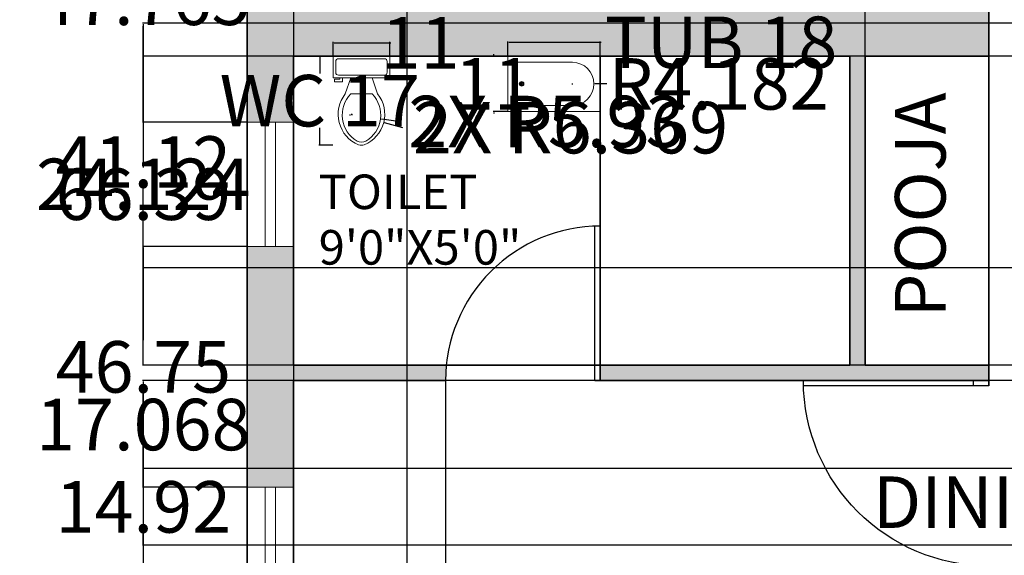
# Model space of a CAD drawing. Units: inches. Extents: x -75 to 484, y -248 to 214.
# Tile 2 of 7: x -29 to 162, y -87 to 17. Entities that reach past the tile are written whole.
import ezdxf

# ---------------------------------------------------------------- set-up
doc = ezdxf.new("R2010")
doc.units = ezdxf.units.IN
doc.header["$MEASUREMENT"] = 0
doc.linetypes.add('ACAD_ISO02W100', pattern=[15, 12, -3])
for name, color, linetype, lineweight in [('A-ANNO-DIMS', 2, 'Continuous', 18), ('A-AREA-IDEN', 7, 'Continuous', 18), ('A-DOOR', 3, 'Continuous', 25), ('A-FLOR-FIXT', 8, 'Continuous', 18), ('A-GLAZ', 4, 'Continuous', 18), ('A-WALL', 7, 'Continuous', 35), ('A-WALL-OVHD', 7, 'ACAD_ISO02W100', 18)]:
    doc.layers.add(name, color=color, linetype=linetype, lineweight=lineweight)
doc.layers.add('A-WALL-PATT', color=252, linetype='Continuous', lineweight=9, true_color=0x939598)
doc.styles.get("Standard").update_dxf_attribs({"font": 'arial.ttf'})
doc.dimstyles.get("Standard").update_dxf_attribs({"dimtxt": 10, "dimasz": 0.18, "dimexe": 0.18, "dimexo": 0.0625, "dimgap": 0.09, "dimtad": 0, "dimtih": 1, "dimtoh": 1, "dimdec": 0, "dimzin": 0, "dimdsep": 46, "dimlunit": 3, "dimtxsty": 'Standard', "dimcen": 0.09, "dimadec": 0, "dimazin": 0, "dimtfac": 1, "dimtdec": 0, "dimtofl": 0, "dimtmove": 0, "dimatfit": 3, "dimfxl": 1, "dimtolj": 1, "dimtzin": 0, "dimarcsym": 0})

# ---------------------------------------------------------------- blocks, each defined once
blk = doc.blocks.new('Toilet - top')
for p, q in [((9.5, -6), (9.5, -2)), ((-10, -8.5), (-8, -8.5)), ((-10, -9.5), (-10, -8.5)), ((-7, -9.5), (-10, -9.5)), ((-8, -8.5), (-8, -8)), ((-7, -8), (-7, -9.5)), ((-4, -8), (-6, -14)), ((4, -8), (6, -14)), ((4, -14), (-4, -14))]:
    blk.add_line(p, q)
blk.add_lwpolyline([(10.5, -8), (10.5, 0), (-10.5, 0), (-10.5, -8)], close=True)
for points in [[(-9.5, -2), (-9.5, -6)], [(8.5, -1), (-8.5, -1)], [(-8.5, -7), (8.5, -7)]]:
    blk.add_lwpolyline(points)
for centre, radius, start, end in [((-8.62, -1.88), 0.884, 81.8699, 188.1301), ((8.62, -1.88), 0.884, 351.8699, 98.1301), ((-8.62, -6.12), 0.884, 171.8699, 278.1301), ((8.62, -6.12), 0.884, 261.8699, 8.1301), ((3.52, -21.58), 12.17, 141.4691, 247.9714), ((4.2, -21.82), 11.33, 136.3677, 238.9468), ((-3.52, -21.58), 12.17, 292.0284, 38.5307), ((-4.2, -21.82), 11.33, 301.053, 43.6321), ((0, -27.88), 4, 245.7318, 294.2682), ((0, -29), 4, 254.8605, 285.1395)]:
    blk.add_arc(centre, radius, start, end)
blk = doc.blocks.new('Bath Tub - 26 x 60 in.')
for p, q in [((8, -18), (10, -18)), ((9, -17), (9, -19))]:
    blk.add_line(p, q)
blk.add_lwpolyline([(0, -36), (0, 0), (60, 0), (60, -36)], close=True)
for points in [[(4, -30), (4, -6)], [(6, -4), (42, -4)], [(42, -32), (6, -32)]]:
    blk.add_lwpolyline(points)
for radius in [1.5, 1]:
    blk.add_circle((9, -18), radius)
for centre, radius, start, end in [((5.75, -5.75), 1.77, 81.8699, 188.1301), ((42, -18), 14, 270, 90), ((5.75, -30.25), 1.77, 171.8699, 278.1301)]:
    blk.add_arc(centre, radius, start, end)
blk = doc.blocks.new('DOOR-SINGLE-36')
for p, q in [((35, 36), (35, 0)), ((36, 36), (36, 0))]:
    blk.add_line(p, q)
blk.add_arc((36, 36), 36, 180, 270)
blk = doc.blocks.new('DOOR-SINGLE-30')
for p, q in [((0, 30), (0, 0)), ((0, 30), (1, 30)), ((1, 30), (1, 0))]:
    blk.add_line(p, q)
blk.add_arc((0, 30), 30, 270, 0)
blk = doc.blocks.new('WIN-48-NOM')
for p, q in [((9, 47.92), (0, 47.92)), ((3.5, 0), (3.5, 47.92)), ((5.5, 0), (5.5, 47.92)), ((0, 0), (9, 0))]:
    blk.add_line(p, q)
blk = doc.blocks.new('*D27')
at = {"layer": 'A-ANNO-DIMS', "color": 0, "lineweight": -2, "transparency": 16777216}
for p, q in [((196.34, -31.46), (182.57, -31.46)), ((182.75, -31.64), (182.75, -71.7)), ((182.75, -122.28), (182.75, -82.22)), ((196.34, -122.46), (182.57, -122.46))]:
    blk.add_line(p, q, dxfattribs=at)
at = {"layer": 'A-ANNO-DIMS', "color": 0, "transparency": 16777216}
for points in [[(182.72, -31.64), (182.78, -31.64), (182.75, -31.46)], [(182.72, -122.28), (182.78, -122.28), (182.75, -122.46)]]:
    blk.add_solid(points, dxfattribs=at)
at = {"layer": 'Defpoints', "color": 0, "transparency": 16777216}
for p in [(196.4, -31.46), (182.75, -122.46), (196.4, -122.46)]:
    blk.add_point(p, dxfattribs=at)
at = {"layer": 'A-ANNO-DIMS', "color": 0, "transparency": 16777216, "insert": (182.75, -76.96), "char_height": 10, "attachment_point": 5}
blk.add_mtext('\\A1;DINING SET 91', dxfattribs=at)
blk = doc.blocks.new('*D29')
at = {"layer": 'A-ANNO-DIMS', "color": 0, "lineweight": -2, "transparency": 16777216}
for p, q in [((31.85, 9.66), (29.14, 9.66)), ((29.32, 9.48), (29.32, 6.27)), ((29.32, -7.46), (29.32, -4.25)), ((31.85, -7.64), (29.14, -7.64))]:
    blk.add_line(p, q, dxfattribs=at)
at = {"layer": 'A-ANNO-DIMS', "color": 0, "transparency": 16777216}
for points in [[(29.29, 9.48), (29.35, 9.48), (29.32, 9.66)], [(29.29, -7.46), (29.35, -7.46), (29.32, -7.64)]]:
    blk.add_solid(points, dxfattribs=at)
at = {"layer": 'Defpoints', "color": 0, "transparency": 16777216}
for p in [(29.32, 9.66), (31.92, 9.66), (31.92, -7.64)]:
    blk.add_point(p, dxfattribs=at)
at = {"layer": 'A-ANNO-DIMS', "color": 0, "transparency": 16777216, "insert": (29.32, 1.01), "char_height": 10, "attachment_point": 5}
blk.add_mtext('\\A1;WC 17', dxfattribs=at)
blk = doc.blocks.new('*D30')
at = {"layer": 'A-ANNO-DIMS', "color": 0, "lineweight": -2, "transparency": 16777216}
for p, q in [((31.92, 9.72), (31.92, 12.43)), ((32.1, 12.25), (42.73, 12.25)), ((42.91, 9.72), (42.91, 12.43)), ((42.91, 12.25), (43.09, 12.25))]:
    blk.add_line(p, q, dxfattribs=at)
at = {"layer": 'A-ANNO-DIMS', "color": 0, "transparency": 16777216}
for points in [[(32.1, 12.28), (32.1, 12.22), (31.92, 12.25)], [(42.73, 12.28), (42.73, 12.22), (42.91, 12.25)]]:
    blk.add_solid(points, dxfattribs=at)
at = {"layer": 'Defpoints', "color": 0, "transparency": 16777216}
for p in [(42.91, 12.25), (31.92, 9.66), (42.91, 9.66)]:
    blk.add_point(p, dxfattribs=at)
at = {"layer": 'A-ANNO-DIMS', "color": 0, "transparency": 16777216, "insert": (48.9, 12.25), "char_height": 10, "attachment_point": 5}
blk.add_mtext('\\A1;11', dxfattribs=at)
blk = doc.blocks.new('*D33')
at = {"layer": 'A-ANNO-DIMS', "color": 0, "lineweight": -2, "transparency": 16777216}
for p, q in [((65.81, 9.72), (65.81, 12.53)), ((65.99, 12.35), (83.56, 12.35)), ((83.74, 9.72), (83.74, 12.53)), ((83.74, 12.35), (83.92, 12.35))]:
    blk.add_line(p, q, dxfattribs=at)
at = {"layer": 'A-ANNO-DIMS', "color": 0, "transparency": 16777216}
for points in [[(65.99, 12.38), (65.99, 12.32), (65.81, 12.35)], [(83.56, 12.38), (83.56, 12.32), (83.74, 12.35)]]:
    blk.add_solid(points, dxfattribs=at)
at = {"layer": 'Defpoints', "color": 0, "transparency": 16777216}
for p in [(83.74, 12.35), (65.81, 9.66), (83.74, 9.66)]:
    blk.add_point(p, dxfattribs=at)
at = {"layer": 'A-ANNO-DIMS', "color": 0, "transparency": 16777216, "insert": (107.22, 12.35), "char_height": 10, "attachment_point": 5}
blk.add_mtext('\\A1;TUB 18', dxfattribs=at)
blk = doc.blocks.new('*D34')
at = {"layer": 'A-ANNO-DIMS', "color": 0, "lineweight": -2, "transparency": 16777216}
for p, q in [((65.75, 9.66), (62.95, 9.66)), ((63.13, 9.84), (63.13, 10.02)), ((65.75, -1.1), (62.95, -1.1)), ((63.13, -1.28), (63.13, -1.46))]:
    blk.add_line(p, q, dxfattribs=at)
at = {"layer": 'A-ANNO-DIMS', "color": 0, "transparency": 16777216}
for points in [[(63.1, 9.84), (63.16, 9.84), (63.13, 9.66)], [(63.1, -1.28), (63.16, -1.28), (63.13, -1.1)]]:
    blk.add_solid(points, dxfattribs=at)
at = {"layer": 'Defpoints', "color": 0, "transparency": 16777216}
for p in [(63.13, 9.66), (65.81, 9.66), (65.81, -1.1)]:
    blk.add_point(p, dxfattribs=at)
at = {"layer": 'A-ANNO-DIMS', "color": 0, "transparency": 16777216, "insert": (63.13, 4.28), "char_height": 10, "attachment_point": 5}
blk.add_mtext('\\A1;11', dxfattribs=at)
blk = doc.blocks.new('*D45')
at = {"layer": 'A-ANNO-DIMS', "color": 0, "lineweight": -2, "transparency": 16777216}
for p, q in [((15.15, 44.59), (-5.12, 44.59)), ((-4.94, 44.41), (-4.94, 25.9)), ((-4.94, -3), (-4.94, 15.51)), ((15.15, -3.18), (-5.12, -3.18))]:
    blk.add_line(p, q, dxfattribs=at)
at = {"layer": 'A-ANNO-DIMS', "color": 0, "transparency": 16777216}
for points in [[(-4.97, 44.41), (-4.91, 44.41), (-4.94, 44.59)], [(-4.97, -3), (-4.91, -3), (-4.94, -3.18)]]:
    blk.add_solid(points, dxfattribs=at)
at = {"layer": 'Defpoints', "color": 0, "transparency": 16777216}
for p in [(15.21, 44.59), (-4.94, -3.18), (15.21, -3.18)]:
    blk.add_point(p, dxfattribs=at)
at = {"layer": 'A-ANNO-DIMS', "color": 0, "transparency": 16777216, "insert": (-4.94, 20.7), "char_height": 10, "attachment_point": 5}
blk.add_mtext('\\A1;47.765', dxfattribs=at)
blk = doc.blocks.new('*D46')
at = {"layer": 'A-ANNO-DIMS', "color": 0, "lineweight": -2, "transparency": 16777216}
for p, q in [((15.15, -3.18), (-5.12, -3.18)), ((-4.94, -3.36), (-4.94, -10.13)), ((-4.94, -27.12), (-4.94, -20.35)), ((15.15, -27.3), (-5.12, -27.3))]:
    blk.add_line(p, q, dxfattribs=at)
at = {"layer": 'A-ANNO-DIMS', "color": 0, "transparency": 16777216}
for points in [[(-4.97, -3.36), (-4.91, -3.36), (-4.94, -3.18)], [(-4.97, -27.12), (-4.91, -27.12), (-4.94, -27.3)]]:
    blk.add_solid(points, dxfattribs=at)
at = {"layer": 'Defpoints', "color": 0, "transparency": 16777216}
for p in [(15.21, -3.18), (-4.94, -27.3), (15.21, -27.3)]:
    blk.add_point(p, dxfattribs=at)
at = {"layer": 'A-ANNO-DIMS', "color": 0, "transparency": 16777216, "insert": (-4.94, -15.24), "char_height": 10, "attachment_point": 5}
blk.add_mtext('\\A1;24.124', dxfattribs=at)
blk = doc.blocks.new('*D47')
at = {"layer": 'A-ANNO-DIMS', "color": 0, "lineweight": -2, "transparency": 16777216}
for p, q in [((15.15, -27.3), (-5.12, -27.3)), ((-4.94, -27.48), (-4.94, -45.48)), ((-4.94, -73.87), (-4.94, -55.87)), ((15.15, -74.05), (-5.12, -74.05))]:
    blk.add_line(p, q, dxfattribs=at)
at = {"layer": 'A-ANNO-DIMS', "color": 0, "transparency": 16777216}
for points in [[(-4.97, -27.48), (-4.91, -27.48), (-4.94, -27.3)], [(-4.97, -73.87), (-4.91, -73.87), (-4.94, -74.05)]]:
    blk.add_solid(points, dxfattribs=at)
at = {"layer": 'Defpoints', "color": 0, "transparency": 16777216}
for p in [(15.21, -27.3), (-4.94, -74.05), (15.21, -74.05)]:
    blk.add_point(p, dxfattribs=at)
at = {"layer": 'A-ANNO-DIMS', "color": 0, "transparency": 16777216, "insert": (-4.94, -50.68), "char_height": 10, "attachment_point": 5}
blk.add_mtext('\\A1;46.75', dxfattribs=at)
blk = doc.blocks.new('*D54')
at = {"layer": 'A-ANNO-DIMS', "color": 0, "lineweight": -2, "transparency": 16777216}
for p, q in [((135.21, -50.28), (135.21, 167.99)), ((135.39, 167.81), (139.89, 167.81)), ((159.03, 167.81), (154.53, 167.81)), ((159.21, -50.28), (159.21, 167.99))]:
    blk.add_line(p, q, dxfattribs=at)
at = {"layer": 'A-ANNO-DIMS', "color": 0, "transparency": 16777216}
for points in [[(135.39, 167.84), (135.39, 167.78), (135.21, 167.81)], [(159.03, 167.84), (159.03, 167.78), (159.21, 167.81)]]:
    blk.add_solid(points, dxfattribs=at)
at = {"layer": 'Defpoints', "color": 0, "transparency": 16777216}
for p in [(159.21, 167.81), (135.21, -50.34), (159.21, -50.34)]:
    blk.add_point(p, dxfattribs=at)
at = {"layer": 'A-ANNO-DIMS', "color": 0, "transparency": 16777216, "insert": (147.21, 167.81), "char_height": 10, "attachment_point": 5}
blk.add_mtext('\\A1;24', dxfattribs=at)
blk = doc.blocks.new('*D58')
at = {"layer": 'A-ANNO-DIMS', "color": 0, "lineweight": -2, "transparency": 16777216}
for p, q in [((24.21, -53.41), (24.21, -241.67)), ((53.74, -53.41), (53.74, -241.67)), ((24.21, -241.49), (24.03, -241.49)), ((53.56, -241.49), (24.39, -241.49))]:
    blk.add_line(p, q, dxfattribs=at)
at = {"layer": 'A-ANNO-DIMS', "color": 0, "transparency": 16777216}
for points in [[(24.39, -241.46), (24.39, -241.52), (24.21, -241.49)], [(53.56, -241.46), (53.56, -241.52), (53.74, -241.49)]]:
    blk.add_solid(points, dxfattribs=at)
at = {"layer": 'Defpoints', "color": 0, "transparency": 16777216}
for p in [(24.21, -53.34), (53.74, -53.34), (24.21, -241.49)]:
    blk.add_point(p, dxfattribs=at)
at = {"layer": 'A-ANNO-DIMS', "color": 0, "transparency": 16777216, "insert": (6.98, -241.49), "char_height": 10, "attachment_point": 5}
blk.add_mtext('\\A1;29.53', dxfattribs=at)
blk = doc.blocks.new('*D60')
at = {"layer": 'A-ANNO-DIMS', "color": 0, "lineweight": -2, "transparency": 16777216}
for p, q in [((375.24, 16.05), (-5.12, 16.05)), ((-4.94, 15.87), (-4.94, -11.95)), ((-4.94, -50.16), (-4.94, -22.35)), ((375.24, -50.34), (-5.12, -50.34))]:
    blk.add_line(p, q, dxfattribs=at)
at = {"layer": 'A-ANNO-DIMS', "color": 0, "transparency": 16777216}
for points in [[(-4.97, 15.87), (-4.91, 15.87), (-4.94, 16.05)], [(-4.97, -50.16), (-4.91, -50.16), (-4.94, -50.34)]]:
    blk.add_solid(points, dxfattribs=at)
at = {"layer": 'Defpoints', "color": 0, "transparency": 16777216}
for p in [(375.3, 16.05), (-4.94, -50.34), (375.3, -50.34)]:
    blk.add_point(p, dxfattribs=at)
at = {"layer": 'A-ANNO-DIMS', "color": 0, "transparency": 16777216, "insert": (-4.94, -17.15), "char_height": 10, "attachment_point": 5}
blk.add_mtext('\\A1;66.39', dxfattribs=at)
blk = doc.blocks.new('*D67')
at = {"layer": 'A-ANNO-DIMS', "color": 0, "lineweight": -2, "transparency": 16777216}
for p, q in [((325.99, -53.34), (-5.12, -53.34)), ((-4.94, -53.52), (-4.94, -56.68)), ((-4.94, -70.23), (-4.94, -67.07)), ((325.99, -70.41), (-5.12, -70.41))]:
    blk.add_line(p, q, dxfattribs=at)
at = {"layer": 'A-ANNO-DIMS', "color": 0, "transparency": 16777216}
for points in [[(-4.97, -53.52), (-4.91, -53.52), (-4.94, -53.34)], [(-4.97, -70.23), (-4.91, -70.23), (-4.94, -70.41)]]:
    blk.add_solid(points, dxfattribs=at)
at = {"layer": 'Defpoints', "color": 0, "transparency": 16777216}
for p in [(326.06, -53.34), (-4.94, -70.41), (326.06, -70.41)]:
    blk.add_point(p, dxfattribs=at)
at = {"layer": 'A-ANNO-DIMS', "color": 0, "transparency": 16777216, "insert": (-4.94, -61.88), "char_height": 10, "attachment_point": 5}
blk.add_mtext('\\A1;17.068', dxfattribs=at)
blk = doc.blocks.new('*D69')
at = {"layer": 'A-ANNO-DIMS', "color": 0, "lineweight": -2, "transparency": 16777216}
for p, q in [((285.15, -53.34), (-5.12, -53.34)), ((-4.94, -53.52), (-4.94, -92.65)), ((-4.94, -142.16), (-4.94, -103.04)), ((285.15, -142.34), (-5.12, -142.34))]:
    blk.add_line(p, q, dxfattribs=at)
at = {"layer": 'A-ANNO-DIMS', "color": 0, "transparency": 16777216}
for points in [[(-4.97, -53.52), (-4.91, -53.52), (-4.94, -53.34)], [(-4.97, -142.16), (-4.91, -142.16), (-4.94, -142.34)]]:
    blk.add_solid(points, dxfattribs=at)
at = {"layer": 'Defpoints', "color": 0, "transparency": 16777216}
for p in [(285.21, -53.34), (-4.94, -142.34), (285.21, -142.34)]:
    blk.add_point(p, dxfattribs=at)
at = {"layer": 'A-ANNO-DIMS', "color": 0, "transparency": 16777216, "insert": (-4.94, -97.84), "char_height": 10, "attachment_point": 5}
blk.add_mtext('\\A1;89', dxfattribs=at)
blk = doc.blocks.new('*D72')
at = {"layer": 'A-ANNO-DIMS', "color": 0, "lineweight": -2, "transparency": 16777216}
for p, q in [((382.5, -70.41), (-5.12, -70.41)), ((-4.94, -70.59), (-4.94, -72.68)), ((-4.94, -85.15), (-4.94, -83.07)), ((382.5, -85.33), (-5.12, -85.33))]:
    blk.add_line(p, q, dxfattribs=at)
at = {"layer": 'A-ANNO-DIMS', "color": 0, "transparency": 16777216}
for points in [[(-4.97, -70.59), (-4.91, -70.59), (-4.94, -70.41)], [(-4.97, -85.15), (-4.91, -85.15), (-4.94, -85.33)]]:
    blk.add_solid(points, dxfattribs=at)
at = {"layer": 'Defpoints', "color": 0, "transparency": 16777216}
for p in [(382.57, -70.41), (-4.94, -85.33), (382.57, -85.33)]:
    blk.add_point(p, dxfattribs=at)
at = {"layer": 'A-ANNO-DIMS', "color": 0, "transparency": 16777216, "insert": (-4.94, -77.87), "char_height": 10, "attachment_point": 5}
blk.add_mtext('\\A1;14.92', dxfattribs=at)
blk = doc.blocks.new('*D76')
at = {"layer": 'A-ANNO-DIMS', "color": 0, "lineweight": -2, "transparency": 16777216}
for p, q in [((24.21, 138.59), (24.21, -241.67)), ((46.2, 104.59), (46.2, -241.67)), ((24.39, -241.49), (46.02, -241.49)), ((46.2, -241.49), (46.38, -241.49))]:
    blk.add_line(p, q, dxfattribs=at)
at = {"layer": 'A-ANNO-DIMS', "color": 0, "transparency": 16777216}
for points in [[(24.39, -241.46), (24.39, -241.52), (24.21, -241.49)], [(46.02, -241.46), (46.02, -241.52), (46.2, -241.49)]]:
    blk.add_solid(points, dxfattribs=at)
at = {"layer": 'Defpoints', "color": 0, "transparency": 16777216}
for p in [(24.21, 138.66), (46.2, 104.66), (46.2, -241.49)]:
    blk.add_point(p, dxfattribs=at)
at = {"layer": 'A-ANNO-DIMS', "color": 0, "transparency": 16777216, "insert": (63.44, -241.49), "char_height": 10, "attachment_point": 5}
blk.add_mtext('\\A1;21.99', dxfattribs=at)
blk = doc.blocks.new('*D77')
at = {"layer": 'A-ANNO-DIMS', "color": 0, "lineweight": -2, "transparency": 16777216}
for p, q in [((159.21, -53.28), (159.21, 167.99)), ((159.39, 167.81), (160.83, 167.81)), ((196.22, 167.81), (194.77, 167.81)), ((196.4, -54.9), (196.4, 167.99))]:
    blk.add_line(p, q, dxfattribs=at)
at = {"layer": 'A-ANNO-DIMS', "color": 0, "transparency": 16777216}
for points in [[(159.39, 167.84), (159.39, 167.78), (159.21, 167.81)], [(196.22, 167.84), (196.22, 167.78), (196.4, 167.81)]]:
    blk.add_solid(points, dxfattribs=at)
at = {"layer": 'Defpoints', "color": 0, "transparency": 16777216}
for p in [(196.4, 167.81), (159.21, -53.34), (196.4, -54.96)]:
    blk.add_point(p, dxfattribs=at)
at = {"layer": 'A-ANNO-DIMS', "color": 0, "transparency": 16777216, "insert": (177.8, 167.81), "char_height": 10, "attachment_point": 5}
blk.add_mtext('\\A1;37.19', dxfattribs=at)
blk = doc.blocks.new('*D78')
at = {"layer": 'A-ANNO-DIMS', "color": 0, "lineweight": -2, "transparency": 16777216}
for p, q in [((240.15, 9.66), (-5.12, 9.66)), ((-4.94, 9.48), (-4.94, -5.79)), ((-4.94, -31.28), (-4.94, -16.01)), ((215.84, -31.46), (-5.12, -31.46))]:
    blk.add_line(p, q, dxfattribs=at)
at = {"layer": 'A-ANNO-DIMS', "color": 0, "transparency": 16777216}
for points in [[(-4.97, 9.48), (-4.91, 9.48), (-4.94, 9.66)], [(-4.97, -31.28), (-4.91, -31.28), (-4.94, -31.46)]]:
    blk.add_solid(points, dxfattribs=at)
at = {"layer": 'Defpoints', "color": 0, "transparency": 16777216}
for p in [(-4.94, 9.66), (240.21, 9.66), (215.9, -31.46)]:
    blk.add_point(p, dxfattribs=at)
at = {"layer": 'A-ANNO-DIMS', "color": 0, "transparency": 16777216, "insert": (-4.94, -10.9), "char_height": 10, "attachment_point": 5}
blk.add_mtext('\\A1;41.12', dxfattribs=at)
blk = doc.blocks.new('*D84')
at = {"layer": 'A-ANNO-DIMS', "color": 0, "lineweight": -2, "transparency": 16777216}
for p, q in [((88.38, 205.37), (88.2, 205.37)), ((88.2, 205.37), (88.2, 132.84)), ((88.2, 11.37), (88.2, 11.55)), ((88.11, 11.46), (88.29, 11.46))]:
    blk.add_line(p, q, dxfattribs=at)
at = {"layer": 'A-ANNO-DIMS', "color": 0, "transparency": 16777216}
blk.add_solid([(88.17, 132.84), (88.23, 132.84), (88.2, 132.66)], dxfattribs=at)
at = {"layer": 'Defpoints', "color": 0, "transparency": 16777216}
for p in [(88.2, 132.66), (88.2, 11.46)]:
    blk.add_point(p, dxfattribs=at)
at = {"layer": 'A-ANNO-DIMS', "color": 0, "transparency": 16777216, "insert": (110.08, 205.37), "char_height": 10, "attachment_point": 5}
blk.add_mtext('\\A1;R121.2', dxfattribs=at)
blk = doc.blocks.new('*D94')
at = {"layer": 'A-ANNO-DIMS', "color": 0, "lineweight": -2, "transparency": 16777216}
for p, q in [((35.48, -1.64), (35.66, -1.64)), ((35.57, -1.73), (35.57, -1.55)), ((45.43, -4.23), (41.9, -3.3))]:
    blk.add_line(p, q, dxfattribs=at)
at = {"layer": 'A-ANNO-DIMS', "color": 0, "transparency": 16777216}
blk.add_solid([(41.91, -3.27), (41.9, -3.33), (41.73, -3.26)], dxfattribs=at)
at = {"layer": 'Defpoints', "color": 0, "transparency": 16777216}
for p in [(35.57, -1.64), (41.73, -3.26)]:
    blk.add_point(p, dxfattribs=at)
at = {"layer": 'A-ANNO-DIMS', "color": 0, "transparency": 16777216, "insert": (78.01, -4.23), "char_height": 10, "attachment_point": 5}
blk.add_mtext('\\A1;2X R6.369', dxfattribs=at)
blk = doc.blocks.new('*D95')
at = {"layer": 'A-ANNO-DIMS', "color": 0, "lineweight": -2, "transparency": 16777216}
for p, q in [((35.12, -1.76), (35.3, -1.76)), ((35.21, -1.85), (35.21, -1.67)), ((44.62, -3.03), (41.27, -2.58))]:
    blk.add_line(p, q, dxfattribs=at)
at = {"layer": 'A-ANNO-DIMS', "color": 0, "transparency": 16777216}
blk.add_solid([(41.27, -2.55), (41.26, -2.61), (41.09, -2.55)], dxfattribs=at)
at = {"layer": 'Defpoints', "color": 0, "transparency": 16777216}
for p in [(35.21, -1.76), (41.09, -2.55)]:
    blk.add_point(p, dxfattribs=at)
at = {"layer": 'A-ANNO-DIMS', "color": 0, "transparency": 16777216, "insert": (73.31, -3.03), "char_height": 10, "attachment_point": 5}
blk.add_mtext('\\A1;2X R5.93', dxfattribs=at)
blk = doc.blocks.new('*D96')
at = {"layer": 'A-ANNO-DIMS', "color": 0, "lineweight": -2, "transparency": 16777216}
for p, q in [((78.27, 4.28), (78.45, 4.28)), ((78.36, 4.19), (78.36, 4.37)), ((85.05, 4.28), (82.72, 4.28))]:
    blk.add_line(p, q, dxfattribs=at)
at = {"layer": 'A-ANNO-DIMS', "color": 0, "transparency": 16777216}
blk.add_solid([(82.72, 4.31), (82.72, 4.25), (82.54, 4.28)], dxfattribs=at)
at = {"layer": 'Defpoints', "color": 0, "transparency": 16777216}
for p in [(78.36, 4.28), (82.54, 4.28)]:
    blk.add_point(p, dxfattribs=at)
at = {"layer": 'A-ANNO-DIMS', "color": 0, "transparency": 16777216, "insert": (106.75, 4.28), "char_height": 10, "attachment_point": 5}
blk.add_mtext('\\A1;R4.182', dxfattribs=at)

msp = doc.modelspace()

# ---------------------------------------------------------------- hatches: boundary and pattern name
at = {"layer": 'A-WALL-PATT'}
h = msp.add_hatch(color=256, dxfattribs=at)
h.dxf.hatch_style = 1
h.paths.add_polyline_path([(184.9004, 147.6567), (15.2094, 147.6567), (15.2094, 92.5031), (24.2094, 92.5031), (24.2094, 138.6567), (186.0436, 138.6567, -0.06325422)])
h.paths.add_polyline_path([(414.2094, 147.6567), (249.2094, 147.6567), (220.9004, 147.6567), (220.9004, 138.6567), (240.2094, 138.6567), (240.2094, 18.6567), (240.2094, 9.6567), (249.2094, 9.6567), (249.2094, 45.6567), (249.2094, 138.6567), (405.2094, 138.6567), (405.2094, 98.3029), (414.2094, 98.3029)])
h.paths.add_polyline_path([(159.2094, 18.6567), (24.2094, 18.6567), (24.2094, 44.5861), (15.2094, 44.5861), (15.2094, 9.6567), (15.2094, -3.1791), (24.2094, -3.1791), (24.2094, 9.6567), (132.2094, 9.6567), (132.2094, -50.3433), (83.7394, -50.3433), (83.7394, -53.3433), (132.2094, -53.3433), (159.2094, -53.3433), (159.2094, -50.3433), (135.2094, -50.3433), (135.2094, 9.6567), (159.2094, 9.6567)])
h.paths.add_polyline_path([(53.8898, -50.3433), (24.2094, -50.3433), (24.2094, -27.303), (15.2094, -27.303), (15.2094, -50.3433), (15.2094, -53.3433), (15.2094, -74.0487), (24.2094, -74.0487), (24.2094, -53.3433), (53.7394, -53.3433, -0.02504709)])
h.paths.add_polyline_path([(24.2094, -121.9657), (15.2094, -121.9657), (15.2094, -212.3433), (15.2094, -221.3433), (24.2094, -221.3433), (84.3017, -221.3433), (84.3017, -212.3433), (24.2094, -212.3433)])
h.paths.add_polyline_path([(414.2094, -155.3433), (414.2094, -53.3433), (414.2094, -50.3433), (414.2094, -36.8417), (405.2094, -36.8417), (405.2094, -50.3433), (309.2094, -50.3433), (309.2094, 16.0463), (324.2573, 16.0463), (324.2573, 18.6567), (284.0663, 18.6567, -0.06325422), (285.2094, 9.6567), (306.2094, 9.6567), (306.2094, -50.3433), (285.2094, -50.3433), (285.2094, -53.3433), (309.2094, -53.3433), (405.2094, -53.3433), (405.2094, -212.3433), (293.2094, -212.3433), (293.2094, -158.3433), (293.2094, -145.3433), (300.0339, -145.3433), (300.0339, -142.3433), (285.2094, -142.3433), (159.2094, -142.3433), (159.2094, -89.3433, -0.02086055), (156.2094, -89.218), (156.2094, -212.3433), (131.9001, -212.3433), (131.9001, -221.3433), (156.2094, -221.3433), (165.2094, -221.3433), (285.2094, -221.3433), (288.6713, -221.3433), (293.2094, -221.3433), (405.2094, -221.3433), (414.2094, -221.3433)])
h.paths.add_polyline_path([(165.2094, -212.3433), (165.2094, -151.3433), (285.2094, -151.3433), (285.2094, -212.3433)], flags=16)
h.paths.add_polyline_path([(189.462, -195.5437), (182.159, -190.2838, -0.23606798), (182.5164, -188.0765), (181.7049, -187.4921), (185.5037, -182.2177), (184.648, -181.6013, -0.04492589), (180.0821, -186.3232), (179.2706, -185.7388), (189.206, -171.9443), (190.0174, -172.5287, -0.04492589), (186.9857, -178.3556), (187.8415, -178.9719), (191.6403, -173.6976), (192.4517, -174.282, -0.23606798), (194.432, -173.2435), (201.735, -178.5034, -0.23606798), (201.3776, -180.7107), (202.189, -181.2952, -0.11764706), (192.2537, -195.0897), (191.4423, -194.5053, -0.23606798)], flags=0)
h.paths.add_polyline_path([(253.751, -177.9543), (254.5293, -177.3263, -0.23606798), (254.0517, -175.1419), (261.056, -169.4904, -0.23606798), (263.0902, -170.419), (263.8684, -169.7911), (267.95, -174.8498), (268.7708, -174.1875, -0.04492589), (265.425, -168.5352), (266.2032, -167.9073), (276.8782, -181.1378), (276.0999, -181.7657, -0.04492589), (271.2826, -177.3006), (270.4618, -177.9629), (274.5434, -183.0216), (273.7651, -183.6495, -0.23606798), (274.2427, -185.834), (267.2383, -191.4854, -0.23606798), (265.2042, -190.5568), (264.4259, -191.1848, -0.11764706)], flags=0)
h.paths.add_polyline_path([(405.2094, -142.3433), (336.0339, -142.3433, -0.02086055), (335.9087, -145.3433), (405.2094, -145.3433)], flags=17)
h.paths.add_polyline_path([(414.2094, 50.4831), (405.2094, 50.4831), (405.2094, 18.6567), (354.2573, 18.6567, -0.02178446), (354.1435, 16.0463), (405.2094, 16.0463), (405.2094, -14.6494), (414.2094, -14.6494), (414.2094, 9.6567)])
h.paths.add_polyline_path([(200.2091, -179.9247), (255.2702, -179.9247), (255.2702, -168.0448), (200.2091, -168.0448)], flags=8)
h.paths.add_polyline_path([(200.2352, -167.6036), (249.7883, -167.6036), (249.7883, -155.8804), (200.2352, -155.8804)], flags=8)

# ---------------------------------------------------------------- linework, layer by layer
at = {"layer": 'A-DOOR'}
for p, q in [((83.7394, -53.3433), (83.7394, -23.3433)), ((159.2094, -53.3433), (123.2094, -53.3433)), ((159.2094, -53.3433), (123.2094, -53.3433)), ((156.2094, -54.3433), (156.2094, -53.3433)), ((159.2094, -53.3433), (159.2094, -54.3433)), ((159.2094, -53.3433), (159.2094, -54.3433)), ((159.2094, -53.3433), (159.2094, -54.3433)), ((159.2094, -53.3433), (159.2094, -54.3433)), ((159.2094, -54.3433), (159.2094, -53.3433))]:
    msp.add_line(p, q, dxfattribs=at)
at = {"layer": 'A-GLAZ'}
for p, q in [((24.2094, -3.1791), (15.2094, -3.1791)), ((18.7094, -27.303), (18.7094, -3.1791)), ((19.7094, -3.1791), (24.2094, -3.1791)), ((20.7094, -27.303), (20.7094, -3.1791)), ((15.2094, -27.303), (24.2094, -27.303))]:
    msp.add_line(p, q, dxfattribs=at)
at = {"layer": 'A-WALL'}
for p, q in [((159.2094, 9.6567), (159.2094, 18.6567)), ((159.2094, 12.9871), (159.2094, 9.6567)), ((15.2094, 9.6567), (15.2094, -50.3433)), ((24.2094, 9.6567), (24.2094, -50.3433)), ((83.7394, -50.3433), (83.7394, 9.6567)), ((132.2094, -50.3433), (132.2094, 9.6567)), ((135.2094, -50.3433), (135.2094, 9.6567)), ((159.2094, 9.6567), (159.2094, -50.3433)), ((15.2094, -53.3433), (15.2094, -48.4472)), ((24.2094, -50.3433), (132.2094, -50.3433)), ((83.7394, -50.3433), (83.7394, -53.3433)), ((159.2094, -50.3433), (135.2094, -50.3433)), ((159.2094, -50.3433), (159.2094, -54.3433)), ((15.2094, -53.3433), (15.2094, -212.3433)), ((24.2094, -53.3433), (53.7394, -53.3433)), ((24.2094, -53.3433), (24.2094, -212.3433)), ((82.7394, -53.3433), (132.2094, -53.3433)), ((159.2094, -53.3433), (132.2094, -53.3433))]:
    msp.add_line(p, q, dxfattribs=at)
for points in [[(249.2094, 147.6567), (15.2094, 147.6567), (15.2094, 9.6567)], [(24.2094, 9.6567), (132.2094, 9.6567)], [(135.2094, 9.6567), (159.2094, 9.6567)]]:
    msp.add_lwpolyline(points, dxfattribs=at)
at = {"layer": 'A-WALL-OVHD'}
msp.add_line((159.2094, 9.6567), (240.2094, 9.6567), dxfattribs=at)

# ---------------------------------------------------------------- block references
at = {"layer": 'A-DOOR', "rotation": 180}
msp.add_blockref('DOOR-SINGLE-30', (83.7394, -23.3433), dxfattribs=at)
at = {"layer": 'A-DOOR', "extrusion": (0, 0, -1), "zscale": -1, "rotation": 90.00000000000014}
msp.add_blockref('DOOR-SINGLE-36', (-123.2094, -89.3433), dxfattribs=at)
at = {"layer": 'A-FLOR-FIXT'}
for name, p, xscale, yscale, zscale in [('Toilet - top', (37.4108, 9.6567), 0.523404442822273, 0.523404442822273, 0.523404442822273), ('Bath Tub - 26 x 60 in.', (65.8148, 9.6567), 0.2987429145537401, 0.2987429145537401, 0.2987429145537401)]:
    msp.add_blockref(name, p, dxfattribs=dict(at, xscale=xscale, yscale=yscale, zscale=zscale))
at = {"layer": 'A-GLAZ', "rotation": 180}
msp.add_blockref('WIN-48-NOM', (24.2094, -74.0487), dxfattribs=at)

# ---------------------------------------------------------------- texts
at = {"layer": 'A-AREA-IDEN'}
msp.add_text('POOJA', height=9.82058, rotation=90, dxfattribs=at).set_placement((150.808, -41.0598))
for s, p in [('TOILET', (29.1054, -20.0424)), ('9\'0"X5\'0"', (29.1054, -30.8228))]:
    msp.add_text(s, height=6.71089, dxfattribs=at).set_placement(p)

# ---------------------------------------------------------------- dimensions: what is measured, and where the dimension line sits
at = {"layer": 'A-ANNO-DIMS'}
for center, mpoint, override, picture, middle in [((88.1998, 11.4599), (88.2, 132.6567), {"dimdec": 1, "dimlfac": 1, "dimrnd": 0, "dimzin": 0, "dimdsep": 46, "dimlunit": 2}, '*D84', (110.0765, 205.3748)), ((78.362, 4.2794), (82.5444, 4.279), {"dimdec": 3, "dimlfac": 1, "dimrnd": 0, "dimzin": 0, "dimdsep": 46, "dimlunit": 2}, '*D96', (85.0538, 4.2788))]:
    dim = msp.add_radius_dim(center=center, mpoint=mpoint, dimstyle='Standard', override=override, dxfattribs=at)
    dim.commit()
    dim.dimension.update_dxf_attribs({"geometry": picture, "text_midpoint": middle, "dimtype": 164})
for base, p1, p2, override, picture, middle in [((159.2094, 167.8067), (135.2094, -50.3433), (159.2094, -50.3433), {"dimdec": 0, "dimlfac": 1, "dimrnd": 0, "dimzin": 0, "dimdsep": 46, "dimlunit": 2}, '*D54', (147.2094, 167.8067)), ((196.3986, 167.8067), (159.2094, -53.3433), (196.3986, -54.9627), {"dimdec": 2, "dimlfac": 1, "dimrnd": 0, "dimzin": 0, "dimdsep": 46, "dimlunit": 2}, '*D77', (177.804, 167.8067)), ((46.1998, -241.4933), (24.2094, 138.6567), (46.1998, 104.6567), {"dimdec": 2, "dimlfac": 1, "dimrnd": 0, "dimzin": 0, "dimdsep": 46, "dimlunit": 2}, '*D76', (63.4378, -241.4933)), ((42.9065, 12.2512), (31.915, 9.6567), (42.9065, 9.6567), {"dimdec": 0, "dimlfac": 1, "dimrnd": 0, "dimzin": 0, "dimdsep": 46, "dimlunit": 2}, '*D30', (48.903, 12.2512)), ((24.2094, -241.4933), (53.7394, -53.3433), (24.2094, -53.3433), {"dimdec": 2, "dimlfac": 1, "dimrnd": 0, "dimzin": 0, "dimdsep": 46, "dimlunit": 2}, '*D58', (6.9817, -241.4933))]:
    dim = msp.add_linear_dim(base=base, p1=p1, p2=p2, dimstyle='Standard', override=override, dxfattribs=at)
    dim.commit()
    dim.dimension.update_dxf_attribs({"geometry": picture, "text_midpoint": middle})
for base, p1, p2, override, picture, middle in [((-4.9406, -3.1791), (15.2094, 44.5861), (15.2094, -3.1791), {"dimdec": 3, "dimlfac": 1, "dimrnd": 0, "dimzin": 0, "dimdsep": 46, "dimlunit": 2}, '*D45', (-4.9406, 20.7035)), ((-4.9406, -50.3433), (375.3026, 16.0463), (375.3026, -50.3433), {"dimdec": 2, "dimlfac": 1, "dimrnd": 0, "dimzin": 0, "dimdsep": 46, "dimlunit": 2}, '*D60', (-4.9406, -17.1485)), ((-4.9406, 9.6567), (215.8986, -31.4627), (240.2094, 9.6567), {"dimdec": 2, "dimlfac": 1, "dimrnd": 0, "dimzin": 0, "dimdsep": 46, "dimlunit": 2}, '*D78', (-4.9406, -10.903)), ((63.1261, 9.6567), (65.8148, -1.098), (65.8148, 9.6567), {"dimdec": 0, "dimlfac": 1, "dimrnd": 0, "dimzin": 0, "dimdsep": 46, "dimlunit": 2}, '*D34', (63.1261, 4.2794)), ((-4.9406, -27.303), (15.2094, -3.1791), (15.2094, -27.303), {"dimdec": 3, "dimlfac": 1, "dimrnd": 0, "dimzin": 0, "dimdsep": 46, "dimlunit": 2}, '*D46', (-4.9406, -15.2411)), ((-4.9406, -74.0487), (15.2094, -27.303), (15.2094, -74.0487), {"dimdec": 2, "dimlfac": 1, "dimrnd": 0, "dimzin": 0, "dimdsep": 46, "dimlunit": 2}, '*D47', (-4.9406, -50.6759)), ((-4.9406, -70.4114), (326.0553, -53.3433), (326.0553, -70.4114), {"dimdec": 3, "dimlfac": 1, "dimrnd": 0, "dimzin": 0, "dimdsep": 46, "dimlunit": 2}, '*D67', (-4.9406, -61.8773)), ((-4.9406, -142.3433), (285.2094, -53.3433), (285.2094, -142.3433), {"dimdec": 0, "dimlfac": 1, "dimrnd": 0, "dimzin": 0, "dimdsep": 46, "dimlunit": 2}, '*D69', (-4.9406, -97.8433)), ((-4.9406, -85.3314), (382.5668, -70.4114), (382.5668, -85.3314), {"dimdec": 2, "dimlfac": 1, "dimrnd": 0, "dimzin": 0, "dimdsep": 46, "dimlunit": 2}, '*D72', (-4.9406, -77.8714))]:
    dim = msp.add_linear_dim(base=base, p1=p1, p2=p2, angle=90, dimstyle='Standard', override=override, dxfattribs=at)
    dim.commit()
    dim.dimension.update_dxf_attribs({"geometry": picture, "text_midpoint": middle})
dim = msp.add_linear_dim(base=(83.7394, 12.3454), p1=(65.8148, 9.6567), p2=(83.7394, 9.6567), text='TUB <>', dimstyle='Standard', override={"dimdec": 0, "dimlfac": 1, "dimrnd": 0, "dimzin": 0, "dimdsep": 46, "dimlunit": 2}, dxfattribs=at)
dim.commit()
dim.dimension.update_dxf_attribs({"geometry": '*D33', "text_midpoint": (107.2188, 12.3454)})
for base, p1, p2, angle, text, picture, middle in [((29.3206, 9.6567), (31.915, -7.6398), (31.915, 9.6567), 90, 'WC <>', '*D29', (29.3206, 1.0085)), ((182.7486, -122.4627), (196.3986, -31.4627), (196.3986, -122.4627), 270, 'DINING SET <>', '*D27', (182.7486, -76.9627))]:
    dim = msp.add_linear_dim(base=base, p1=p1, p2=p2, angle=angle, text=text, dimstyle='Standard', override={"dimdec": 0, "dimlfac": 1, "dimrnd": 0, "dimzin": 0, "dimdsep": 46, "dimlunit": 2}, dxfattribs=at)
    dim.commit()
    dim.dimension.update_dxf_attribs({"geometry": picture, "text_midpoint": middle})
for center, mpoint, override, picture, middle in [((35.2125, -1.7626), (41.0894, -2.553), {"dimdec": 2, "dimlfac": 1, "dimrnd": 0, "dimzin": 0, "dimdsep": 46, "dimlunit": 2}, '*D95', (44.6155, -3.0273)), ((35.5687, -1.6386), (41.7289, -3.257), {"dimdec": 3, "dimlfac": 1, "dimrnd": 0, "dimzin": 0, "dimdsep": 46, "dimlunit": 2}, '*D94', (45.4251, -4.228))]:
    dim = msp.add_radius_dim(center=center, mpoint=mpoint, text='2X <>', dimstyle='Standard', override=override, dxfattribs=at)
    dim.commit()
    dim.dimension.update_dxf_attribs({"geometry": picture, "text_midpoint": middle, "dimtype": 164})

doc.saveas('drawing.dxf')
